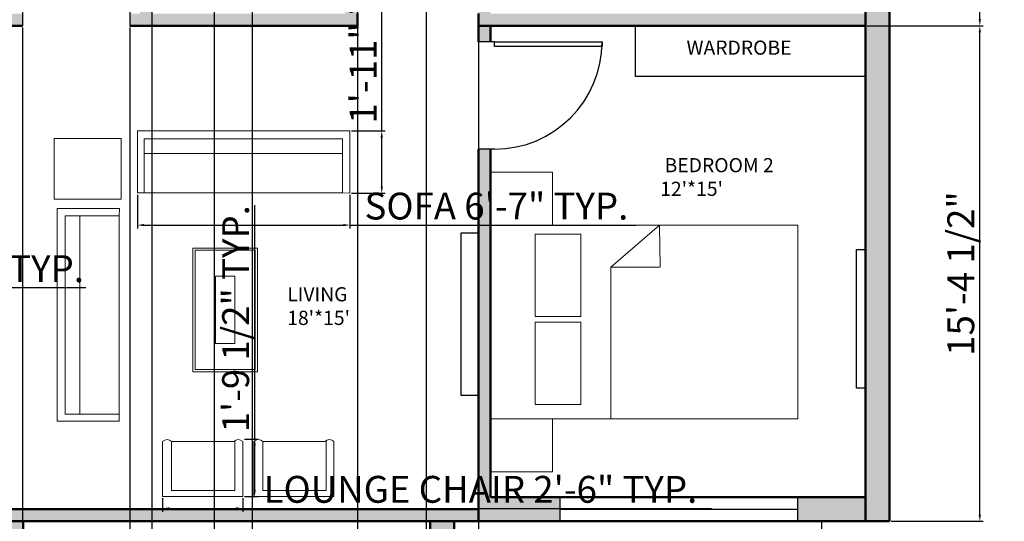
# Model space of a CAD drawing. Units: inches. Extents: x 772 to 1415, y 1573 to 2261.
# Tile 3 of 4: x 984 to 1350, y 1820 to 2007. Entities that reach past the tile are written whole.
import ezdxf

# ---------------------------------------------------------------- set-up
doc = ezdxf.new("R2010")
doc.units = ezdxf.units.IN
for name, color, linetype, lineweight in [('A-ANNO-DIMS', 2, 'Continuous', 18), ('A-ANNO-TEXT', 10, 'Continuous', 25), ('A-AREA-IDEN', 10, 'Continuous', 25), ('A-FLOR-EDGE', 7, 'Continuous', 25), ('A-FURN-FIXD', 210, 'Continuous', 25), ('A-WALL-PATT', 140, 'Continuous', 13), ('DOOR', 52, 'Continuous', 25), ('FUR', 210, 'Continuous', 18), ('WALL', 7, 'Continuous', 50), ('WINDOW', 80, 'Continuous', 25)]:
    doc.layers.add(name, color=color, linetype=linetype, lineweight=lineweight)
doc.styles.get("Standard").update_dxf_attribs({"font": 'arial.ttf'})
doc.dimstyles.new('ISO-25', dxfattribs={"dimtxt": 10, "dimasz": 2.5, "dimexe": 1.25, "dimexo": 0.625, "dimtad": 1, "dimdec": 0, "dimlunit": 4, "dimtxsty": 'Standard', "dimcen": 2.5, "dimadec": 0, "dimazin": 0, "dimtfac": 1, "dimtdec": 0, "dimtmove": 0, "dimatfit": 3, "dimfxl": 1, "dimarcsym": 0})

# ---------------------------------------------------------------- blocks, each defined once
blk = doc.blocks.new('*U2')
for p, q in [((0, 0), (0, -6)), ((40, 0), (40, -6))]:
    blk.add_line(p, q)
blk.add_lwpolyline([(0, 0), (0, 40), (1.75, 40), (1.75, 0)], close=True)
blk.add_arc((0, 0), 40, 0, 90)
blk = doc.blocks.new('CHAIR-LOUNGE')
for p, q in [((0, 20.45), (0, 0)), ((26.89, 20.45), (26.11, 20.45)), ((29.8, 0), (29.8, 20.45)), ((0, 0), (29.8, 0))]:
    blk.add_line(p, q)
blk.add_lwpolyline([(3.35, 2.16), (26.89, 2.16), (26.89, 20.45), (3.35, 20.45)], close=True)
for centre in [(1.67, 18.73), (28.12, 18.73)]:
    blk.add_arc(centre, 2.4, 45.7795, 134.2205)
blk = doc.blocks.new('SOFA')
for p, q in [((0, 0.2), (0, 23.2)), ((0, 23.2), (79.09, 23.2)), ((79.09, 23.2), (79.09, 0)), ((2.52, 14.84), (76.36, 14.84)), ((2.52, 0.2), (0, 0.2)), ((79.09, 0), (76.36, 0.2))]:
    blk.add_line(p, q)
blk.add_lwpolyline([(2.52, 20.23), (76.36, 20.23), (76.36, 0.2), (2.52, 0.2)], close=True)
blk = doc.blocks.new('WIN-88IN')
blk.add_line((0, 4.5), (88.26, 4.5))
blk.add_lwpolyline([(0, 9), (88.26, 9), (88.26, 0), (0, 0)], close=True)
blk = doc.blocks.new('*D26')
at = {"layer": 'A-ANNO-DIMS', "color": 0, "lineweight": -2, "transparency": 16777216}
for p, q in [((926.29, 1907.91), (926.29, 1905.75)), ((928.79, 1907), (933.54, 1907)), ((936.04, 1907.91), (936.04, 1905.75)), ((936.04, 1907), (1008.52, 1907))]:
    blk.add_line(p, q, dxfattribs=at)
at = {"layer": 'A-ANNO-DIMS', "color": 0, "transparency": 16777216}
for points in [[(928.79, 1907.42), (928.79, 1906.58), (926.29, 1907)], [(933.54, 1907.42), (933.54, 1906.58), (936.04, 1907)]]:
    blk.add_solid(points, dxfattribs=at)
at = {"layer": 'Defpoints', "color": 0, "transparency": 16777216}
for p in [(926.29, 1908.53), (936.04, 1908.53), (936.04, 1907)]:
    blk.add_point(p, dxfattribs=at)
at = {"layer": 'A-ANNO-DIMS', "color": 0, "transparency": 16777216, "insert": (973.53, 1912.73), "char_height": 10, "attachment_point": 5}
blk.add_mtext('0\'-10" TYP.', dxfattribs=at)
blk = doc.blocks.new('*D27')
at = {"layer": 'A-ANNO-DIMS', "color": 0, "lineweight": -2, "transparency": 16777216}
for p, q in [((1037.11, 1828.64), (1037.11, 1823.55)), ((1066.91, 1828.64), (1066.91, 1823.55)), ((1039.61, 1824.8), (1064.41, 1824.8)), ((1066.91, 1824.8), (1241.4, 1824.8))]:
    blk.add_line(p, q, dxfattribs=at)
at = {"layer": 'A-ANNO-DIMS', "color": 0, "transparency": 16777216}
for points in [[(1039.61, 1825.21), (1039.61, 1824.38), (1037.11, 1824.8)], [(1064.41, 1825.21), (1064.41, 1824.38), (1066.91, 1824.8)]]:
    blk.add_solid(points, dxfattribs=at)
at = {"layer": 'Defpoints', "color": 0, "transparency": 16777216}
for p in [(1037.11, 1829.27), (1066.91, 1829.27), (1066.91, 1824.8)]:
    blk.add_point(p, dxfattribs=at)
at = {"layer": 'A-ANNO-DIMS', "color": 0, "transparency": 16777216, "insert": (1155.4, 1830.59), "char_height": 10, "attachment_point": 5}
blk.add_mtext('LOUNGE CHAIR 2\'-6" TYP.', dxfattribs=at)
blk = doc.blocks.new('*D28')
at = {"layer": 'A-ANNO-DIMS', "color": 0, "lineweight": -2, "transparency": 16777216}
for p, q in [((1071.38, 1850.62), (1071.38, 1937.68)), ((1067.53, 1850.62), (1072.63, 1850.62)), ((1071.38, 1831.77), (1071.38, 1848.12)), ((1067.53, 1829.27), (1072.63, 1829.27))]:
    blk.add_line(p, q, dxfattribs=at)
at = {"layer": 'A-ANNO-DIMS', "color": 0, "transparency": 16777216}
for points in [[(1070.96, 1848.12), (1071.8, 1848.12), (1071.38, 1850.62)], [(1070.96, 1831.77), (1071.8, 1831.77), (1071.38, 1829.27)]]:
    blk.add_solid(points, dxfattribs=at)
at = {"layer": 'Defpoints', "color": 0, "transparency": 16777216}
for p in [(1066.91, 1850.62), (1071.38, 1850.62), (1066.91, 1829.27)]:
    blk.add_point(p, dxfattribs=at)
at = {"layer": 'A-ANNO-DIMS', "color": 0, "transparency": 16777216, "insert": (1065.58, 1895.4), "char_height": 10, "attachment_point": 5, "rotation": 90}
blk.add_mtext('1\'-9 1/2" TYP.', dxfattribs=at)
blk = doc.blocks.new('*D29')
at = {"layer": 'A-ANNO-DIMS', "color": 0, "lineweight": -2, "transparency": 16777216}
for p, q in [((1027.72, 1941.49), (1027.72, 1929.01)), ((1106.81, 1941.49), (1106.81, 1929.01)), ((1030.22, 1930.26), (1104.31, 1930.26)), ((1106.81, 1930.26), (1213.38, 1930.26))]:
    blk.add_line(p, q, dxfattribs=at)
at = {"layer": 'A-ANNO-DIMS', "color": 0, "transparency": 16777216}
for points in [[(1030.22, 1930.67), (1030.22, 1929.84), (1027.72, 1930.26)], [(1104.31, 1930.67), (1104.31, 1929.84), (1106.81, 1930.26)]]:
    blk.add_solid(points, dxfattribs=at)
at = {"layer": 'Defpoints', "color": 0, "transparency": 16777216}
for p in [(1027.72, 1942.12), (1106.81, 1942.12), (1106.81, 1930.26)]:
    blk.add_point(p, dxfattribs=at)
at = {"layer": 'A-ANNO-DIMS', "color": 0, "transparency": 16777216, "insert": (1161.34, 1936.05), "char_height": 10, "attachment_point": 5}
blk.add_mtext('SOFA 6\'-7" TYP.', dxfattribs=at)
blk = doc.blocks.new('*D30')
at = {"layer": 'A-ANNO-DIMS', "color": 0, "lineweight": -2, "transparency": 16777216}
for p, q in [((1118.67, 1965.32), (1118.67, 2036.85)), ((1107.43, 1965.32), (1119.92, 1965.32)), ((1118.67, 1944.62), (1118.67, 1962.82)), ((1107.43, 1942.12), (1119.92, 1942.12))]:
    blk.add_line(p, q, dxfattribs=at)
at = {"layer": 'A-ANNO-DIMS', "color": 0, "transparency": 16777216}
for points in [[(1118.25, 1962.82), (1119.09, 1962.82), (1118.67, 1965.32)], [(1118.25, 1944.62), (1119.09, 1944.62), (1118.67, 1942.12)]]:
    blk.add_solid(points, dxfattribs=at)
at = {"layer": 'Defpoints', "color": 0, "transparency": 16777216}
for p in [(1106.81, 1965.32), (1118.67, 1965.32), (1106.81, 1942.12)]:
    blk.add_point(p, dxfattribs=at)
at = {"layer": 'A-ANNO-DIMS', "color": 0, "transparency": 16777216, "insert": (1113.02, 2002.34), "char_height": 10, "attachment_point": 5, "rotation": 90}
blk.add_mtext('1\'-11" TYP.', dxfattribs=at)
blk = doc.blocks.new('*D46')
at = {"layer": 'A-ANNO-DIMS', "color": 0, "lineweight": -2, "transparency": 16777216}
for p, q in [((1299.28, 2004.48), (1342.5, 2004.48)), ((1341.25, 1822.48), (1341.25, 2001.98)), ((1308.28, 1819.98), (1342.5, 1819.98))]:
    blk.add_line(p, q, dxfattribs=at)
at = {"layer": 'A-ANNO-DIMS', "color": 0, "transparency": 16777216}
for points in [[(1340.83, 2001.98), (1341.67, 2001.98), (1341.25, 2004.48)], [(1340.83, 1822.48), (1341.67, 1822.48), (1341.25, 1819.98)]]:
    blk.add_solid(points, dxfattribs=at)
at = {"layer": 'Defpoints', "color": 0, "transparency": 16777216}
for p in [(1298.65, 2004.48), (1341.25, 2004.48), (1307.65, 1819.98)]:
    blk.add_point(p, dxfattribs=at)
at = {"layer": 'A-ANNO-DIMS', "color": 0, "transparency": 16777216, "insert": (1335.46, 1912.23), "char_height": 10, "attachment_point": 5, "rotation": 90}
blk.add_mtext('15\'-4 1/2"', dxfattribs=at)
blk = doc.blocks.new('*D47')
at = {"layer": 'A-ANNO-DIMS', "color": 0, "lineweight": -2, "transparency": 16777216}
for p, q in [((1308.28, 2185.98), (1342.5, 2185.98)), ((1341.25, 2006.98), (1341.25, 2183.48)), ((1299.28, 2004.48), (1342.5, 2004.48))]:
    blk.add_line(p, q, dxfattribs=at)
at = {"layer": 'A-ANNO-DIMS', "color": 0, "transparency": 16777216}
for points in [[(1340.83, 2183.48), (1341.67, 2183.48), (1341.25, 2185.98)], [(1340.83, 2006.98), (1341.67, 2006.98), (1341.25, 2004.48)]]:
    blk.add_solid(points, dxfattribs=at)
at = {"layer": 'Defpoints', "color": 0, "transparency": 16777216}
for p in [(1307.65, 2185.98), (1341.25, 2185.98), (1298.65, 2004.48)]:
    blk.add_point(p, dxfattribs=at)
at = {"layer": 'A-ANNO-DIMS', "color": 0, "transparency": 16777216, "insert": (1335.46, 2095.23), "char_height": 10, "attachment_point": 5, "rotation": 90}
blk.add_mtext('15\'-1 1/2"', dxfattribs=at)
blk = doc.blocks.new('*D59')
at = {"layer": 'A-ANNO-DIMS', "color": 0, "lineweight": -2, "transparency": 16777216}
for p, q in [((1109.65, 2003.86), (1109.65, 1580.94)), ((1154.65, 2003.86), (1154.65, 1580.94)), ((1112.15, 1582.19), (1152.15, 1582.19))]:
    blk.add_line(p, q, dxfattribs=at)
at = {"layer": 'A-ANNO-DIMS', "color": 0, "transparency": 16777216}
for points in [[(1112.15, 1582.61), (1112.15, 1581.78), (1109.65, 1582.19)], [(1152.15, 1582.61), (1152.15, 1581.78), (1154.65, 1582.19)]]:
    blk.add_solid(points, dxfattribs=at)
at = {"layer": 'Defpoints', "color": 0, "transparency": 16777216}
for p in [(1109.65, 2004.48), (1154.65, 2004.48), (1154.65, 1582.19)]:
    blk.add_point(p, dxfattribs=at)
at = {"layer": 'A-ANNO-DIMS', "color": 0, "transparency": 16777216, "insert": (1132.15, 1587.93), "char_height": 10, "attachment_point": 5}
blk.add_mtext('3\'-9"', dxfattribs=at)
blk = doc.blocks.new('*D60')
at = {"layer": 'A-ANNO-DIMS', "color": 0, "lineweight": -2, "transparency": 16777216}
for p, q in [((984.95, 2003.86), (984.95, 1580.94)), ((1024.95, 2003.86), (1024.95, 1580.94)), ((987.45, 1582.19), (1022.45, 1582.19))]:
    blk.add_line(p, q, dxfattribs=at)
at = {"layer": 'A-ANNO-DIMS', "color": 0, "transparency": 16777216}
for points in [[(987.45, 1582.61), (987.45, 1581.78), (984.95, 1582.19)], [(1022.45, 1582.61), (1022.45, 1581.78), (1024.95, 1582.19)]]:
    blk.add_solid(points, dxfattribs=at)
at = {"layer": 'Defpoints', "color": 0, "transparency": 16777216}
for p in [(984.95, 2004.48), (1024.95, 2004.48), (1024.95, 1582.19)]:
    blk.add_point(p, dxfattribs=at)
at = {"layer": 'A-ANNO-DIMS', "color": 0, "transparency": 16777216, "insert": (1004.95, 1587.93), "char_height": 10, "attachment_point": 5}
blk.add_mtext('3\'-4"', dxfattribs=at)
blk = doc.blocks.new('*D61')
at = {"layer": 'A-ANNO-DIMS', "color": 0, "lineweight": -2, "transparency": 16777216}
for p, q in [((1033.15, 2008.36), (1033.15, 1580.94)), ((1056.25, 2011.79), (1056.25, 1580.94)), ((1035.65, 1582.19), (1053.75, 1582.19)), ((1056.25, 1582.19), (1093.41, 1582.19))]:
    blk.add_line(p, q, dxfattribs=at)
at = {"layer": 'A-ANNO-DIMS', "color": 0, "transparency": 16777216}
for points in [[(1035.65, 1582.61), (1035.65, 1581.78), (1033.15, 1582.19)], [(1053.75, 1582.61), (1053.75, 1581.78), (1056.25, 1582.19)]]:
    blk.add_solid(points, dxfattribs=at)
at = {"layer": 'Defpoints', "color": 0, "transparency": 16777216}
for p in [(1056.25, 2012.41), (1033.15, 2008.98), (1056.25, 1582.19)]:
    blk.add_point(p, dxfattribs=at)
at = {"layer": 'A-ANNO-DIMS', "color": 0, "transparency": 16777216, "insert": (1076.08, 1587.84), "char_height": 10, "attachment_point": 5}
blk.add_mtext('1\'-11"', dxfattribs=at)
blk = doc.blocks.new('*D62')
at = {"layer": 'A-ANNO-DIMS', "color": 0, "lineweight": -2, "transparency": 16777216}
for p, q in [((1033.15, 2092.36), (1033.15, 1580.94)), ((1070.44, 2092.36), (1070.44, 1580.94)), ((1035.65, 1582.19), (1067.94, 1582.19)), ((1070.44, 1582.19), (1124.06, 1582.19))]:
    blk.add_line(p, q, dxfattribs=at)
at = {"layer": 'A-ANNO-DIMS', "color": 0, "transparency": 16777216}
for points in [[(1035.65, 1582.61), (1035.65, 1581.78), (1033.15, 1582.19)], [(1067.94, 1582.61), (1067.94, 1581.78), (1070.44, 1582.19)]]:
    blk.add_solid(points, dxfattribs=at)
at = {"layer": 'Defpoints', "color": 0, "transparency": 16777216}
for p in [(1033.15, 2092.98), (1070.44, 2092.98), (1070.44, 1582.19)]:
    blk.add_point(p, dxfattribs=at)
at = {"layer": 'A-ANNO-DIMS', "color": 0, "transparency": 16777216, "insert": (1098.5, 1587.99), "char_height": 10, "attachment_point": 5}
blk.add_mtext('3\'-1 1/2"', dxfattribs=at)
blk = doc.blocks.new('*D63')
at = {"layer": 'A-ANNO-DIMS', "color": 0, "lineweight": -2, "transparency": 16777216}
for p, q in [((1109.65, 2099.86), (1109.65, 1580.94)), ((1135.17, 2099.86), (1135.17, 1580.94)), ((1112.15, 1582.19), (1132.67, 1582.19)), ((1135.17, 1582.19), (1188.98, 1582.19))]:
    blk.add_line(p, q, dxfattribs=at)
at = {"layer": 'A-ANNO-DIMS', "color": 0, "transparency": 16777216}
for points in [[(1112.15, 1582.61), (1112.15, 1581.78), (1109.65, 1582.19)], [(1132.67, 1582.61), (1132.67, 1581.78), (1135.17, 1582.19)]]:
    blk.add_solid(points, dxfattribs=at)
at = {"layer": 'Defpoints', "color": 0, "transparency": 16777216}
for p in [(1109.65, 2100.48), (1135.17, 2100.48), (1135.17, 1582.19)]:
    blk.add_point(p, dxfattribs=at)
at = {"layer": 'A-ANNO-DIMS', "color": 0, "transparency": 16777216, "insert": (1163.33, 1587.99), "char_height": 10, "attachment_point": 5}
blk.add_mtext('2\'-1 1/2"', dxfattribs=at)

msp = doc.modelspace()

# ---------------------------------------------------------------- hatches: boundary and pattern name
at = {"layer": 'A-WALL-PATT'}
h = msp.add_hatch(color=256, dxfattribs=at)
h.dxf.hatch_style = 1
h.paths.add_polyline_path([(885.72, 2185.98), (827.65, 2185.98), (827.65, 1992.85), (836.65, 1992.85), (836.65, 2176.98), (885.72, 2176.98)])
h.paths.add_polyline_path([(1050.98, 2185.98), (977.81, 2185.98), (977.81, 2176.98), (1028.65, 2176.98), (1050.98, 2176.98)])
h.paths.add_polyline_path([(1112.88, 2185.98), (1085.61, 2185.98), (1085.61, 2176.98), (1105.15, 2176.98), (1112.88, 2176.98)])
h.paths.add_polyline_path([(1192.68, 2185.98), (1147.51, 2185.98), (1147.51, 2176.98), (1181.65, 2176.98), (1192.68, 2176.98)])
h.paths.add_polyline_path([(1307.65, 2185.98), (1284.78, 2185.98), (1284.78, 2176.98), (1298.65, 2176.98), (1298.65, 1819.98), (1307.65, 1819.98)])
h.paths.add_polyline_path([(1033.15, 2176.98), (1028.65, 2176.98), (1028.65, 2036.41), (1032.25, 2036.41, -0.009373), (1033.15, 2036.4)])
h.paths.add_polyline_path([(1036.22, 2092.98), (1033.15, 2092.98), (1033.15, 2088.48), (1036.22, 2088.48)])
h.paths.add_polyline_path([(1154.65, 2104.98), (1135.16, 2104.98, -0.008763), (1135.17, 2104.13), (1135.17, 2100.48), (1154.65, 2100.48)])
h.paths.add_polyline_path([(1159.15, 2176.98), (1154.65, 2176.98), (1154.65, 2051.78), (1159.15, 2051.78)])
h.paths.add_polyline_path([(914.37, 1839.72), (927.25, 1839.72), (927.25, 1850.6), (914.37, 1850.6)], flags=9)
h.paths.add_polyline_path([(1081.37, 1890.08), (1108.45, 1890.08), (1108.45, 1909.77), (1081.37, 1909.77)], flags=9)
h.paths.add_polyline_path([(1220.18, 1938.14), (1269.92, 1938.14), (1269.92, 1957.83), (1220.18, 1957.83)], flags=9)
h.paths.add_polyline_path([(1219.66, 2046.23), (1263.24, 2046.23), (1263.24, 2065.92), (1219.66, 2065.92)], flags=9)
h.paths.add_polyline_path([(1107.96, 2127.66), (1143.78, 2127.66), (1143.78, 2147.35), (1107.96, 2147.35)], flags=9)
h.paths.add_polyline_path([(1040.84, 2046.02), (1081.99, 2046.02), (1081.99, 2065.72), (1040.84, 2065.72)], flags=9)
h.paths.add_polyline_path([(1051.44, 2131.75), (1073.61, 2131.75), (1073.61, 2151.44), (1051.44, 2151.44)], flags=9)
h.paths.add_polyline_path([(953.87, 2096.26), (1003.05, 2096.26), (1003.05, 2115.95), (953.87, 2115.95)], flags=9)
h = msp.add_hatch(color=256, dxfattribs=at)
h.dxf.hatch_style = 1
h.paths.add_polyline_path([(1109.65, 2176.98), (1105.15, 2176.98), (1105.15, 2092.98), (1072.93, 2092.98), (1070.44, 2092.98), (1070.44, 2088.48), (1105.15, 2088.48), (1105.15, 2008.98), (1093.16, 2008.98), (1033.15, 2008.98), (1033.15, 2012.41), (1032.25, 2012.41), (1028.65, 2012.41), (1028.65, 2008.98), (1024.95, 2008.98), (1024.95, 2004.48), (1033.15, 2004.48), (1109.65, 2004.48), (1109.65, 2008.98), (1109.65, 2088.48)])
h.paths.add_polyline_path([(1159.15, 1958.53), (1154.65, 1958.53), (1154.65, 1819.98), (1185.12, 1819.98), (1185.12, 1828.98), (1159.15, 1828.98)])
h.paths.add_polyline_path([(1298.65, 1828.98), (1273.39, 1828.98), (1273.39, 1819.98), (1298.65, 1819.98)])
h.paths.add_polyline_path([(1107.96, 2127.66), (1143.78, 2127.66), (1143.78, 2147.35), (1107.96, 2147.35)], flags=9)
h = msp.add_hatch(color=256, dxfattribs=at)
h.dxf.hatch_style = 1
h.paths.add_polyline_path([(836.65, 1835.78), (827.65, 1835.78), (827.65, 1770.04), (833.65, 1770.04), (836.65, 1770.04)])
h.paths.add_polyline_path([(1154.65, 1824.48), (938.65, 1824.48), (836.65, 1824.48), (836.65, 1819.98), (980.65, 1819.98), (1154.65, 1819.98)])
h.paths.add_polyline_path([(836.65, 1962.89), (827.65, 1962.89), (827.65, 1865.74), (836.65, 1865.74)])
h.paths.add_polyline_path([(913.15, 1980.86), (910.62, 1980.86, -0.029352), (908.65, 1980.98), (908.65, 1968.98), (900.27, 1968.98), (855.22, 1968.98), (855.22, 1964.48), (913.15, 1964.48)])
h.paths.add_polyline_path([(855.22, 1968.98), (836.65, 1968.98), (836.65, 1964.48), (855.22, 1964.48)])
h.paths.add_polyline_path([(984.95, 2008.98), (836.65, 2008.98), (836.65, 2004.48), (908.65, 2004.48), (984.95, 2004.48)])
h.paths.add_polyline_path([(1298.65, 2008.98), (1171.7, 2008.98), (1154.65, 2008.98), (1154.65, 2004.48), (1298.65, 2004.48)])
h.paths.add_polyline_path([(1159.15, 2011.78), (1154.65, 2011.78), (1154.65, 2008.98), (1159.15, 2008.98)])
h.paths.add_polyline_path([(1159.15, 2004.48), (1154.65, 2004.48), (1154.65, 1998.53), (1159.15, 1998.53)])
h = msp.add_hatch(color=256, dxfattribs=at)
h.dxf.hatch_style = 1
h.paths.add_polyline_path([(863.4, 1654.98), (836.65, 1654.98), (836.65, 1678.98), (836.65, 1730.15, -0.01877), (833.65, 1730.04), (827.65, 1730.04), (827.65, 1645.98), (863.4, 1645.98)])
h.paths.add_polyline_path([(985.15, 1654.98), (985.15, 1819.98), (976.15, 1819.98), (976.15, 1654.98), (951.66, 1654.98), (951.66, 1645.98), (985.15, 1645.98)])
h.paths.add_polyline_path([(989, 1737.48), (989, 1740.48), (985.15, 1740.48), (985.15, 1731.48), (989, 1731.48)])
h.paths.add_polyline_path([(1045.2, 1740.48), (1028.89, 1740.48, -0.01877), (1029, 1737.48), (1029, 1731.48), (1045.2, 1731.48)])
h.paths.add_polyline_path([(1145.65, 1819.98), (1136.65, 1819.98), (1136.65, 1740.48), (1133.46, 1740.48), (1133.46, 1731.48), (1145.65, 1731.48)])

# ---------------------------------------------------------------- linework, layer by layer
at = {"layer": 'A-FLOR-EDGE'}
msp.add_line((1282.31, 1819.98), (1282.31, 1657.99), dxfattribs=at)
at = {"layer": 'A-FURN-FIXD'}
for points in [[(1213.13, 2004.48), (1298.65, 2004.48), (1298.65, 1985.6), (1213.13, 1985.6)], [(1154.65, 1927.29), (1148.11, 1927.29), (1148.11, 1866.97), (1154.65, 1866.97)], [(1298.65, 1869.56), (1295.34, 1869.56), (1295.34, 1921.14), (1298.65, 1921.14)]]:
    msp.add_lwpolyline(points, close=True, dxfattribs=at)
at = {"layer": 'FUR'}
for p, q in [((1222.03, 1930.27), (1203.96, 1914.64)), ((1222.31, 1914.64), (1222.03, 1930.27)), ((1203.96, 1858.12), (1203.96, 1914.64)), ((1203.96, 1914.64), (1222.03, 1914.64))]:
    msp.add_line(p, q, dxfattribs=at)
for points in [[(996.69, 1939.93), (1021.74, 1939.93), (1021.74, 1962.56), (996.69, 1962.56)], [(1159.15, 1930.27), (1182.26, 1930.27), (1182.26, 1950), (1159.15, 1950)], [(1159.15, 1858.12), (1273.49, 1858.12), (1273.49, 1930.27), (1159.15, 1930.27)], [(1175.73, 1896.28), (1192.81, 1896.28), (1192.81, 1926.93), (1175.73, 1926.93)], [(1048.38, 1921.69), (1072.43, 1921.69), (1072.43, 1875.68), (1048.38, 1875.68)], [(1049.2, 1920.87), (1071.61, 1920.87), (1071.61, 1876.5), (1049.2, 1876.5)], [(1056.85, 1911.24), (1063.93, 1911.24), (1063.93, 1886.13), (1056.85, 1886.13)], [(1175.73, 1863.5), (1192.81, 1863.5), (1192.81, 1894.15), (1175.73, 1894.15)], [(1159.15, 1838.39), (1182.26, 1838.39), (1182.26, 1858.12), (1159.15, 1858.12)]]:
    msp.add_lwpolyline(points, close=True, dxfattribs=at)
at = {"layer": 'WALL'}
for p, q in [((1307.65, 2185.98), (1307.65, 1819.98)), ((1298.65, 2176.98), (1298.65, 1819.98)), ((1109.65, 2008.98), (1109.65, 2004.48)), ((1154.65, 2008.98), (1154.65, 2004.48)), ((984.95, 2004.48), (836.65, 2004.48)), ((1033.15, 2004.48), (1024.95, 2004.48)), ((1033.15, 2004.48), (1109.65, 2004.48)), ((1154.65, 2004.48), (1298.65, 2004.48)), ((1154.65, 2004.48), (1154.65, 1998.53)), ((1159.15, 2004.48), (1159.15, 1998.53)), ((1298.65, 2004.48), (1298.65, 1824.48)), ((1154.65, 1958.53), (1154.65, 1819.98)), ((1159.15, 1958.53), (1159.15, 1828.98)), ((1159.15, 1828.98), (1298.65, 1828.98)), ((1154.65, 1824.48), (938.65, 1824.48)), ((1154.65, 1819.98), (836.65, 1819.98)), ((985.15, 1819.98), (985.15, 1654.98)), ((985.15, 1819.98), (985.15, 1735.98)), ((1136.65, 1740.48), (1136.65, 1819.98)), ((1145.65, 1731.48), (1145.65, 1819.98)), ((1154.65, 1819.98), (1298.65, 1819.98)), ((1298.65, 1819.98), (1307.65, 1819.98))]:
    msp.add_line(p, q, dxfattribs=at)

# ---------------------------------------------------------------- block references
at = {"layer": 'DOOR', "xscale": -1}
msp.add_blockref('*U2', (1024.95, 2010.48), dxfattribs=at)
at = {"layer": 'DOOR', "rotation": 270}
msp.add_blockref('*U2', (1160.65, 1998.53), dxfattribs=at)
at = {"layer": 'FUR'}
for name, p in [('SOFA', (1027.72, 1942.12)), ('CHAIR-LOUNGE', (1037.11, 1829.26)), ('CHAIR-LOUNGE', (1071.05, 1829.26))]:
    msp.add_blockref(name, p, dxfattribs=at)
at = {"layer": 'FUR', "rotation": 90.0000000000001}
msp.add_blockref('SOFA', (1021.08, 1857.3), dxfattribs=at)
at = {"layer": 'WINDOW'}
msp.add_blockref('WIN-88IN', (1185.12, 1819.98), dxfattribs=at)

# ---------------------------------------------------------------- texts
at = {"layer": 'A-ANNO-TEXT', "insert": (1232.09, 1998.96), "char_height": 5.277, "attachment_point": 1}
msp.add_mtext_dynamic_manual_height_columns('WARDROBE', width=83.1931, gutter_width=26.39, heights=[0], dxfattribs=at)
at = {"layer": 'A-AREA-IDEN', "char_height": 5.277, "attachment_point": 1}
for s, insert in [(" BEDROOM 2\\P12'*15'", (1222.31, 1955.21)), ("LIVING\\P18'*15'", (1083.49, 1907.15))]:
    msp.add_mtext_dynamic_manual_height_columns(s, width=83.1931, gutter_width=26.39, heights=[0], dxfattribs=dict(at, insert=insert))

# ---------------------------------------------------------------- dimensions: what is measured, and where the dimension line sits
at = {"layer": 'A-ANNO-DIMS'}
for base, p1, p2, picture, middle in [((1341.25, 2185.98), (1298.65, 2004.48), (1307.65, 2185.98), '*D47', (1335.46, 2095.23)), ((1341.25, 2004.48), (1307.65, 1819.98), (1298.65, 2004.48), '*D46', (1335.46, 1912.23))]:
    dim = msp.add_linear_dim(base=base, p1=p1, p2=p2, angle=90, dimstyle='ISO-25', override={"dimdec": 1, "dimlfac": 1, "dimrnd": 0, "dimzin": 1, "dimdsep": 46, "dimlunit": 4, "dimfrac": 2}, dxfattribs=at)
    dim.commit()
    dim.dimension.update_dxf_attribs({"geometry": picture, "text_midpoint": middle})
for base, p1, p2, picture, middle in [((1135.17, 1582.19), (1109.65, 2100.48), (1135.17, 2100.48), '*D63', (1163.33, 1587.99)), ((1070.44, 1582.19), (1033.15, 2092.98), (1070.44, 2092.98), '*D62', (1098.5, 1587.99)), ((1056.25, 1582.19), (1033.15, 2008.98), (1056.25, 2012.41), '*D61', (1076.08, 1587.84)), ((1024.95, 1582.19), (984.95, 2004.48), (1024.95, 2004.48), '*D60', (1004.95, 1587.93)), ((1154.65, 1582.19), (1109.65, 2004.48), (1154.65, 2004.48), '*D59', (1132.15, 1587.93))]:
    dim = msp.add_linear_dim(base=base, p1=p1, p2=p2, dimstyle='ISO-25', override={"dimdec": 1, "dimlfac": 1, "dimrnd": 0, "dimzin": 1, "dimdsep": 46, "dimlunit": 4, "dimfrac": 2}, dxfattribs=at)
    dim.commit()
    dim.dimension.update_dxf_attribs({"geometry": picture, "text_midpoint": middle})
for base, p1, p2, angle, picture, middle in [((1118.67, 1965.32), (1106.81, 1942.12), (1106.81, 1965.32), 90, '*D30', (1113.02, 2002.34)), ((1071.379, 1850.6168), (1066.9094, 1829.265), (1066.9094, 1850.6168), 90, '*D28', (1065.5835, 1895.3994)), ((936.0429, 1906.9998), (926.2923, 1908.5349), (936.0429, 1908.5349), 0, '*D26', (973.5302, 1912.7305))]:
    dim = msp.add_linear_dim(base=base, p1=p1, p2=p2, angle=angle, text='<> TYP.', dimstyle='ISO-25', override={"dimdec": 1, "dimlfac": 1, "dimrnd": 0, "dimzin": 1, "dimdsep": 46, "dimlunit": 4, "dimfrac": 2}, dxfattribs=at)
    dim.commit()
    dim.dimension.update_dxf_attribs({"geometry": picture, "text_midpoint": middle})
for base, p1, p2, text, picture, middle in [((1106.81, 1930.26), (1027.72, 1942.12), (1106.81, 1942.12), 'SOFA <> TYP.', '*D29', (1161.34, 1936.05)), ((1066.91, 1824.8), (1037.11, 1829.27), (1066.91, 1829.27), 'LOUNGE CHAIR <> TYP.', '*D27', (1155.4, 1830.59))]:
    dim = msp.add_linear_dim(base=base, p1=p1, p2=p2, text=text, dimstyle='ISO-25', override={"dimdec": 1, "dimlfac": 1, "dimrnd": 0, "dimzin": 1, "dimdsep": 46, "dimlunit": 4, "dimfrac": 2}, dxfattribs=at)
    dim.commit()
    dim.dimension.update_dxf_attribs({"geometry": picture, "text_midpoint": middle})

doc.saveas('drawing.dxf')
